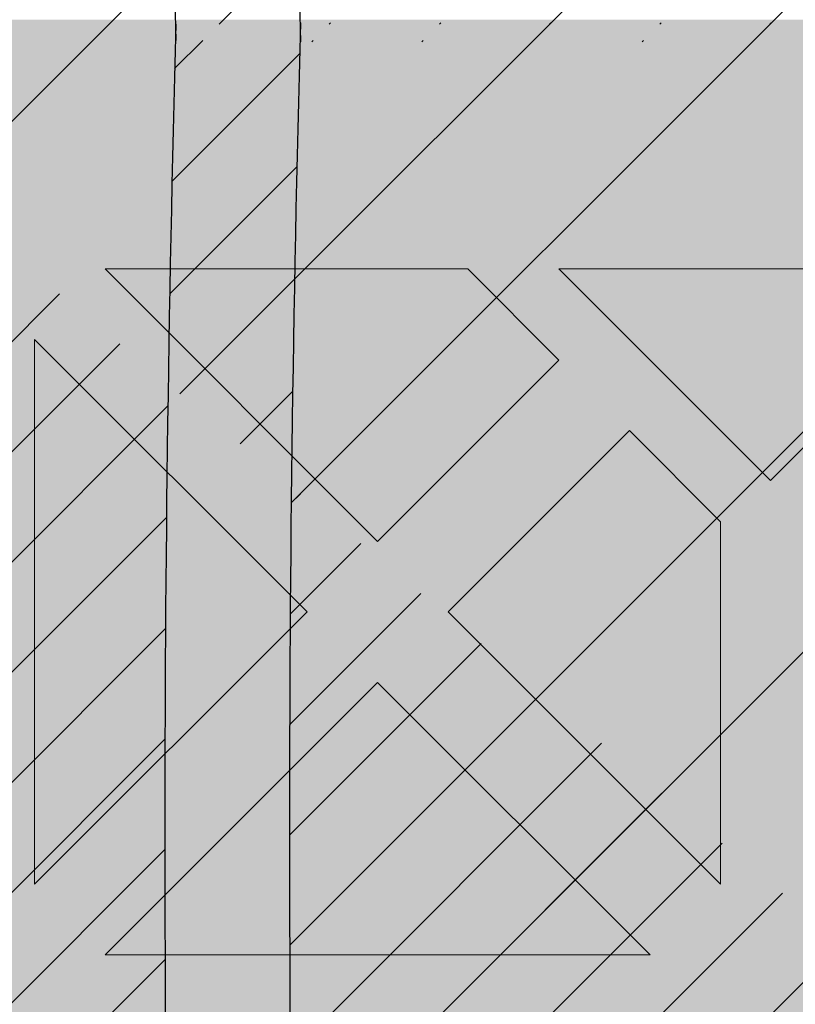
# Model space of a CAD drawing. Units: inches. Extents: x 844 to 2234, y 346 to 1084.
# Tile 11 of 93: x 1120.937 to 1122.921, y 693.702 to 696.22. Entities that reach past the tile are written whole.
import ezdxf

# ---------------------------------------------------------------- set-up
doc = ezdxf.new("R2010")
doc.units = ezdxf.units.IN
doc.header["$MEASUREMENT"] = 0
for name, color, linetype, lineweight in [('A-ANNO-DIMS', 2, 'Continuous', 18), ('furniture', 8, 'Continuous', 18), ('RA-AP-01$0$INT', 35, 'Continuous', 5)]:
    doc.layers.add(name, color=color, linetype=linetype, lineweight=lineweight)
doc.layers.add('RA-AP-01$0$FURN', color=3, linetype='Continuous')
doc.layers.add('RA-AP-01$0$WOOD', color=64, linetype='Continuous')
doc.styles.get("Standard").update_dxf_attribs({"font": 'arial.ttf'})
doc.dimstyles.get("Standard").update_dxf_attribs({"dimtxt": 6, "dimasz": 3, "dimexe": 0.18, "dimexo": 0.0625, "dimgap": 0.09, "dimtad": 0, "dimtih": 1, "dimtoh": 1, "dimdec": 1, "dimzin": 0, "dimdsep": 46, "dimlunit": 3, "dimtxsty": 'Standard', "dimblk": 'ARCHTICK', "dimcen": 0.09, "dimadec": 0, "dimazin": 0, "dimtfac": 1, "dimtdec": 1, "dimtofl": 0, "dimtmove": 0, "dimatfit": 3, "dimfxl": 1, "dimtolj": 1, "dimtzin": 0, "dimarcsym": 0})

# ---------------------------------------------------------------- blocks, each defined once
blk = doc.blocks.new('A$C18D01794')
at = {"layer": 'RA-AP-01$0$INT'}
h = blk.add_hatch(color=256, dxfattribs=at)
h.paths.add_polyline_path([(4.585917135068448, -6.356712009588273), (4.614201406330596, -6.356712009589021), (4.668846067270487, -6.411356670531338), (4.723490728212344, -6.356712009591912), (4.771774999457151, -6.35671200959319), (4.826419660396886, -6.411356670535356), (4.862780050090322, -6.374996280843536), (4.844495778842715, -6.356712009595112), (4.862780050090411, -6.356712009595595), (4.905206456960182, -6.399138416468211), (4.947632863832445, -6.356712009597838), (4.965917135079675, -6.356712009598322), (4.947632863831759, -6.374996280845421), (4.983993253523576, -6.411356670538857), (5.038637914464627, -6.356712009600247), (5.08692218571208, -6.356712009601523), (5.141566846649976, -6.411356670541852), (5.196211507589851, -6.356712009604411), (5.224495778822615, -6.356712009605161), (4.905206456953975, -6.676001331473793)])
h.paths.add_polyline_path([(4.895206456956031, -6.637717060225675), (4.895206456958921, -6.528427738347902), (4.840561796018589, -6.583072399285802)], flags=16)
h.paths.add_polyline_path([(4.915206456955638, -6.637717060226121), (4.969851117895509, -6.583072399288678), (4.915206456957609, -6.528427738348344)], flags=16)
h.paths.add_polyline_path([(4.826419660395175, -6.568930263661755), (4.881064321335613, -6.514285602723745), (4.771774999456703, -6.514285602720857)], flags=16)
h.paths.add_polyline_path([(4.983993253519558, -6.568930263665262), (5.038637914460456, -6.514285602726792), (4.929348592581548, -6.514285602724816)], flags=16)
h.paths.add_polyline_path([(4.881064321336025, -6.494285602723742), (4.826419660397532, -6.439640941782821), (4.771774999457062, -6.494285602720859)], flags=16)
h.paths.add_polyline_path([(4.929348592582019, -6.494285602724817), (5.038637914460982, -6.494285602726792), (4.983993253522945, -6.439640941786327)], flags=16)
h.paths.add_polyline_path([(4.895206456960191, -6.480143467100443), (4.895206456962115, -6.407422687715913), (4.876922185715016, -6.389138416467584), (4.840561796021581, -6.425498806159401)], flags=16)
h.paths.add_polyline_path([(4.915206456958487, -6.480143467100889), (4.969851117899527, -6.425498806162279), (4.933490728206909, -6.389138416468043), (4.9152064569598, -6.40742268771434)], flags=16)
h.paths.add_polyline_path([(4.757632863832376, -6.480143467096812), (4.812277524772842, -6.425498806158772), (4.757632863834348, -6.370854145217844)], flags=16)
h.paths.add_polyline_path([(4.737632863832376, -6.480143467096286), (4.737632863834348, -6.370854145217375), (4.682988202893906, -6.425498806155385)], flags=16)
h.paths.add_polyline_path([(5.05278005008503, -6.480143467103376), (5.052780050087917, -6.370854145224413), (4.998135389146995, -6.425498806162908)], flags=16)
h.paths.add_polyline_path([(5.072780050085024, -6.480143467103744), (5.127424711025931, -6.42549880616527), (5.072780050087916, -6.370854145224832)], flags=16)
h.paths.add_polyline_path([(4.935917135072783, -6.706712009592292), (5.255206456948811, -6.387422687716309), (5.255206456948932, -6.415706958964177), (5.200561796010279, -6.470351619902839), (5.255206456949403, -6.524996280841948), (5.25520645694961, -6.5732805520894), (5.200561796009787, -6.627925213029239), (5.236922185702417, -6.664285602721864), (5.255206456949919, -6.646001331474357), (5.255206456949998, -6.664285602721898), (5.212780050078687, -6.706712009592262), (5.25520645695036, -6.749138416463932), (5.255206456950438, -6.767422687711313), (5.236922185702424, -6.749138416463297), (5.200561796009796, -6.785498806155928), (5.255206456950753, -6.840143467096874), (5.25520645695096, -6.888427738341682), (5.200561796010322, -6.943072399282328), (5.255206456951428, -6.997717060223427), (5.255206456951547, -7.026001331471006)])
h.paths.add_polyline_path([(5.042988202883395, -6.785498806155427), (5.097632863823085, -6.840143467095101), (5.097632863822622, -6.730854145216193)], flags=16)
h.paths.add_polyline_path([(5.028846067259663, -6.771356670531693), (5.083490728198774, -6.716712009592573), (4.974201406321001, -6.716712009593042)], flags=16)
h.paths.add_polyline_path([(5.117632863823087, -6.840143467095186), (5.172277524762331, -6.785498806155926), (5.11763286382262, -6.730854145216225)], flags=16)
h.paths.add_polyline_path([(5.08349072819877, -6.696712009593886), (5.028846067259652, -6.642067348654775), (4.974201406320998, -6.696712009593438)], flags=16)
h.paths.add_polyline_path([(5.131774999446817, -6.854285602718917), (5.186419660386065, -6.799640941779662), (5.241064321325782, -6.854285602719365)], flags=17)
h.paths.add_polyline_path([(5.131774999446228, -6.716712009592374), (5.186419660386065, -6.771356670532194), (5.222780050079488, -6.734996280838764), (5.204495778832781, -6.716712009592063)], flags=16)
h.paths.add_polyline_path([(5.097632863822613, -6.682569873970264), (5.097632863823061, -6.573280552091354), (5.042988202883383, -6.627925213031044)], flags=16)
h.paths.add_polyline_path([(5.131774999446899, -6.874285602718915), (5.241064321325809, -6.874285602719364), (5.186419660386591, -6.928930263658598)], flags=17)
h.paths.add_polyline_path([(5.131774999446226, -6.696712009594078), (5.204495778830767, -6.696712009594374), (5.22278005007868, -6.67842773834687), (5.186419660386049, -6.642067348654249)], flags=16)
h.paths.add_polyline_path([(5.11763286382262, -6.682569873970225), (5.17227752476232, -6.627925213030515), (5.117632863823064, -6.573280552091267)], flags=16)
h.paths.add_polyline_path([(5.186419660386069, -6.613783077405491), (5.241064321325754, -6.559138416465795), (5.131774999446791, -6.559138416466263)], flags=16)
h.paths.add_polyline_path([(5.131774999446872, -6.539138416466263), (5.24106432132578, -6.539138416465794), (5.186419660386554, -6.484493755526573)], flags=16)
h.paths.add_polyline_path([(5.255206456951811, -7.08742268770861), (5.255206456951895, -7.106712009588038), (4.555206456956052, -7.106712009588038), (4.555206456956136, -7.087422687708617), (4.905206456953973, -6.737422687710788)])
h.paths.add_polyline_path([(4.983993253513404, -6.8444937555241), (4.92934859257295, -6.899138416462108), (5.03863791445186, -6.899138416465014)], flags=16)
h.paths.add_polyline_path([(4.969851117889988, -6.83035161990006), (4.915206456952556, -6.775706958960171), (4.915206456949648, -6.884996280837944)], flags=16)
h.paths.add_polyline_path([(4.929348592572535, -6.919138416462105), (4.983993253511019, -6.973783077403037), (5.038637914451496, -6.919138416465012)], flags=16)
h.paths.add_polyline_path([(5.052780050074912, -6.93328055208906), (4.998135389134438, -6.987925213027088), (5.052780050072919, -7.042569873968025)], flags=16)
h.paths.add_polyline_path([(5.07278005007491, -6.933280552089588), (5.072780050072918, -7.042569873968497), (5.127424711013374, -6.987925213030498)], flags=16)
h.paths.add_polyline_path([(4.89520645695295, -6.775706958959721), (4.840561796013067, -6.830351619897157), (4.895206456950961, -6.884996280837494)], flags=16)
h.paths.add_polyline_path([(4.915206456948365, -6.933280552085403), (4.915206456946434, -7.006001331471951), (4.933490728192729, -7.024285602719066), (4.969851117886972, -6.987925213026453)], flags=16)
h.paths.add_polyline_path([(4.881064321327021, -6.899138416461022), (4.82641966038902, -6.84449375552057), (4.771774999448108, -6.899138416459029)], flags=16)
h.paths.add_polyline_path([(4.895206456950073, -6.933280552084951), (4.840561796009022, -6.987925213023558), (4.876922185700835, -7.024285602716997), (4.895206456948749, -7.006001331469487)], flags=16)
h.paths.add_polyline_path([(4.983993253510392, -7.0020673486505), (4.947632863816944, -7.038427738342319), (4.965917135064043, -7.05671200959023), (5.038637914448995, -7.056712009591555)], flags=16)
h.paths.add_polyline_path([(4.881064321326543, -6.91913841646102), (4.771774999447578, -6.919138416459031), (4.826419660385607, -6.973783077399508)], flags=16)
h.paths.add_polyline_path([(4.905206456946447, -7.014285602717636), (4.862780050074785, -7.056712009588352), (4.947632863816685, -7.056712009589775)], flags=16)
h.paths.add_polyline_path([(5.14156684663679, -7.002067348654549), (5.086922185696452, -7.056712009592438), (5.196211507574223, -7.056712009594425)], flags=16)
h.paths.add_polyline_path([(4.8264196603837, -7.002067348646972), (4.771774999442643, -7.056712009585575), (4.8444957788276, -7.056712009587508), (4.862780050075511, -7.038427738340416)], flags=16)
h.paths.add_polyline_path([(4.812277524760289, -6.98792521302292), (4.757632863822258, -6.933280552082447), (4.757632863819352, -7.042569873961408)], flags=16)
h.paths.add_polyline_path([(4.73763286382226, -6.933280552082079), (4.682988202881349, -6.987925213020536), (4.737632863819352, -7.04256987396099)], flags=16)
h.paths.add_polyline_path([(4.723490728195188, -7.056712009584289), (4.668846067257299, -7.002067348643949), (4.614201406317417, -7.056712009581383)], flags=16)
h.paths.add_polyline_path([(4.597632863829262, -6.706712009592262), (4.555206456957951, -6.664285602721896), (4.555206456958029, -6.646001331474357), (4.573490728205535, -6.664285602721864), (4.609851117898167, -6.627925213029238), (4.555206456958338, -6.573280552089402), (4.555206456958546, -6.524996280841952), (4.60985111789767, -6.470351619902839), (4.555206456959015, -6.415706958964177), (4.555206456959138, -6.387422687716309), (4.874495778835167, -6.70671200959229), (4.5552064569564, -7.026001331471015), (4.555206456956523, -6.997717060223433), (4.609851117897629, -6.94307239928233), (4.555206456956988, -6.888427738341681), (4.555206456957198, -6.840143467096881), (4.609851117898153, -6.78549880615593), (4.573490728205528, -6.749138416463297), (4.555206456957507, -6.76742268771132), (4.555206456957585, -6.749138416463933)])
h.paths.add_polyline_path([(4.712780050085332, -6.730854145216195), (4.712780050084863, -6.840143467095105), (4.767424711024555, -6.785498806155427)], flags=16)
h.paths.add_polyline_path([(4.726922185709173, -6.716712009592573), (4.781566846648288, -6.771356670531693), (4.836211507586949, -6.716712009593043)], flags=16)
h.paths.add_polyline_path([(4.692780050085327, -6.730854145216225), (4.638135389145619, -6.785498806155928), (4.692780050084865, -6.840143467095185)], flags=16)
h.paths.add_polyline_path([(4.726922185709182, -6.696712009593886), (4.836211507586949, -6.696712009593436), (4.7815668466483, -6.642067348654773)], flags=16)
h.paths.add_polyline_path([(4.678637914461726, -6.71671200959237), (4.605917135075169, -6.716712009592063), (4.587632863828464, -6.734996280838766), (4.623993253521887, -6.771356670532195)], flags=16)
h.paths.add_polyline_path([(4.712780050085336, -6.68256987397026), (4.767424711024568, -6.627925213031042), (4.71278005008489, -6.573280552091352)], flags=16)
h.paths.add_polyline_path([(4.678637914461726, -6.696712009594076), (4.623993253521899, -6.642067348654247), (4.587632863829271, -6.67842773834687), (4.605917135077185, -6.696712009594376)], flags=16)
h.paths.add_polyline_path([(4.692780050085336, -6.682569873970228), (4.692780050084889, -6.573280552091267), (4.638135389145632, -6.627925213030515)], flags=16)
h.paths.add_polyline_path([(4.623993253521885, -6.799640941779662), (4.678637914461131, -6.854285602718915), (4.56934859258217, -6.854285602719365)], flags=17)
h.paths.add_polyline_path([(4.623993253521901, -6.613783077405509), (4.678637914461158, -6.559138416466263), (4.569348592582195, -6.559138416465795)], flags=16)
h.paths.add_polyline_path([(4.678637914461051, -6.874285602718915), (4.623993253521361, -6.928930263658598), (4.569348592582143, -6.874285602719364)], flags=17)
h.paths.add_polyline_path([(4.678637914461076, -6.539138416466263), (4.623993253521399, -6.484493755526573), (4.569348592582167, -6.539138416465796)], flags=16)
h = blk.add_hatch(color=256, dxfattribs=at)
h.paths.add_polyline_path([(4.895206456952951, -6.77570695895972), (4.840561796013068, -6.830351619897156), (4.895206456950958, -6.884996280837495)])
h.paths.add_polyline_path([(4.915206456949649, -6.884996280837942), (4.969851117889987, -6.830351619900054), (4.915206456952556, -6.775706958960171)])
h.paths.add_polyline_path([(5.038637914451862, -6.899138416465013), (4.983993253513403, -6.8444937555241), (4.929348592572953, -6.899138416462106)])
h.paths.add_polyline_path([(4.929348592572535, -6.919138416462105), (4.983993253511018, -6.973783077403037), (5.038637914451497, -6.919138416465012)])
h.paths.add_polyline_path([(4.915206456948366, -6.933280552085397), (4.915206456946433, -7.006001331471951), (4.93349072819273, -7.024285602719068), (4.969851117886972, -6.987925213026454)])
h.paths.add_polyline_path([(5.038637914448995, -7.056712009591553), (4.983993253510389, -7.002067348650502), (4.947632863816946, -7.038427738342318), (4.965917135064043, -7.05671200959023)])
h.paths.add_polyline_path([(5.05278005007292, -7.042569873968023), (5.05278005007491, -6.933280552089059), (4.998135389134438, -6.987925213027088)])
h.paths.add_polyline_path([(5.07278005007292, -7.042569873968496), (5.127424711013374, -6.987925213030498), (5.072780050074909, -6.933280552089588)])
h.paths.add_polyline_path([(5.141566846636789, -7.002067348654547), (5.086922185696449, -7.056712009592438), (5.196211507574223, -7.056712009594425)])
h.paths.add_polyline_path([(4.947632863816688, -7.056712009589774), (4.905206456946449, -7.014285602717634), (4.862780050074784, -7.056712009588353)])
h.paths.add_polyline_path([(4.840561796009025, -6.987925213023556), (4.876922185700834, -7.024285602716997), (4.895206456948747, -7.006001331469488), (4.895206456950075, -6.933280552084953)])
h.paths.add_polyline_path([(4.88106432132654, -6.919138416461021), (4.771774999447577, -6.919138416459031), (4.826419660385606, -6.973783077399508)])
h.paths.add_polyline_path([(4.881064321327019, -6.899138416461022), (4.826419660389019, -6.844493755520571), (4.771774999448108, -6.89913841645903)])
h.paths.add_polyline_path([(4.757632863819352, -7.042569873961409), (4.812277524760284, -6.987925213022922), (4.757632863822259, -6.933280552082447)])
h.paths.add_polyline_path([(4.8264196603837, -7.002067348646974), (4.771774999442646, -7.056712009585575), (4.844495778827599, -7.05671200958751), (4.862780050075512, -7.038427738340417)])
h.paths.add_polyline_path([(4.737632863819352, -7.042569873960988), (4.737632863822258, -6.933280552082078), (4.682988202881349, -6.987925213020538)])
h.paths.add_polyline_path([(4.668846067257299, -7.002067348643952), (4.61420140631742, -7.056712009581384), (4.723490728195189, -7.056712009584292)])
for p, q in [((4.771774999447578, -6.919138416459031), (4.881064321326541, -6.919138416461022)), ((4.771774999447578, -6.919138416459031), (4.826419660385606, -6.973783077399508)), ((4.881064321326541, -6.919138416461022), (4.826419660385606, -6.973783077399508)), ((4.757632863822258, -6.933280552082445), (4.812277524760285, -6.987925213022922)), ((4.757632863822258, -6.933280552082445), (4.757632863819352, -7.042569873961408)), ((4.895206456950073, -6.933280552084951), (4.840561796009024, -6.987925213023556)), ((4.895206456948748, -7.006001331469903), (4.895206456950073, -6.933280552084951)), ((4.757632863819352, -7.042569873961408), (4.812277524760285, -6.987925213022922)), ((4.840561796009024, -6.987925213023554), (4.876922185700835, -7.024285602716997)), ((4.771774999442645, -7.056712009585574), (4.8264196603837, -7.002067348646972)), ((4.826419660383698, -7.002067348646972), (4.862780050075511, -7.038427738340416)), ((4.895206456946431, -7.006001331471805), (4.876922185700835, -7.024285602716997)), ((4.905206456946449, -7.014285602717635), (4.862780050074783, -7.056712009588354)), ((4.905206456946449, -7.014285602717635), (4.94763286381669, -7.056712009589775)), ((4.844495778827597, -7.056712009587512), (4.862780050075513, -7.038427738340416)), ((4.844495778827597, -7.05671200958751), (4.771774999442645, -7.056712009585574)), ((4.94763286381669, -7.056712009589775), (4.862780050074783, -7.056712009588354))]:
    blk.add_line(p, q, dxfattribs=at)
blk = doc.blocks.new('A$C32926AE1')
at = {"layer": 'RA-AP-01$0$FURN'}
h = blk.add_hatch(dxfattribs=at)
h.set_pattern_fill('ANSI31', color=256, scale=0.1, style=0)
h.set_pattern_definition([(45, (0, 0), (-0.0088388347648318, 0.0088388347648318), [])])
edge = h.paths.add_edge_path(flags=16)
edge.add_arc((4.904771284329206, 4.246793130718756), 0.2603971832811541, 75.22398030683196, 104.7760196931204)
edge.add_arc((4.904771284329206, 4.246793130718756), 0.2603971832811541, 75.223980306832, 104.77601969312039, ccw=False)
edge = h.paths.add_edge_path(flags=16)
edge.add_arc((4.904771284329206, 4.067062675376612), 0.2603971832811541, 255.2239803068796, 284.776019693168)
edge.add_arc((4.904771284329206, 4.067062675376612), 0.2603971832811541, 255.22398030687958, 284.77601969316805, ccw=False)
edge = h.paths.add_edge_path(flags=0)
edge.add_arc((4.904771284329206, 4.067062675376612), 0.2603971832811541, 255.2239803068796, 284.776019693168)
edge.add_arc((4.904771284329206, 4.067062675376612), 0.2603971832811541, 255.22398030687958, 284.77601969316805, ccw=False)
edge = h.paths.add_edge_path(flags=0)
edge.add_arc((4.904771284329206, 4.067062675376612), 0.2603971832811541, 255.2239803068796, 284.776019693168)
edge.add_arc((4.904771284329206, 4.067062675376612), 0.2603971832811541, 255.22398030687958, 284.77601969316805, ccw=False)
edge = h.paths.add_edge_path()
edge.add_arc((4.604388392048174, 4.588829985554312), 0.1599999999999918, 342.3781640246255, 354.4317409793762)
edge.add_arc((5.090145208887507, 4.43216705527679), 0.3503971832811637, 162.0091218307731, 180.3186872093483)
edge.add_arc((5.205154176610243, 4.588829985554953), 0.1599999999999917, 185.5682590208461, 197.6218359767349)
edge.add_arc((4.904771284329229, 4.246793130718735), 0.3503971832811761, 72.00912183053516, 107.9908781690354)
edge.add_arc((9.535952835716557, 4.28682295566602), 4.798342501046485, 178.2875002453811, 181.5576802719453)
edge.add_arc((4.719397359771122, 4.43216705527679), 0.3503971832811637, 359.6813127906516, 377.9908781692269)
edge.add_arc((9.535967292294904, 4.286822350292874), 4.778371420254705, 178.2965938931842, 181.5667745797229)
edge.add_arc((4.719397359771122, 4.43216705527679), 0.3303971832811637, 359.6813127906516, 377.9908781692269)
edge.add_arc((0.2735752763637294, 4.286822350292874), 4.7783714202547, 358.4332254202771, 361.7034061068158)
edge.add_arc((5.061434214606998, 4.732549947558029), 0.1600000000000254, 252.3781640250584, 264.4317409792362)
edge.add_arc((4.748108354051257, 4.732549947558012), 0.1600000000000541, 275.5682590208426, 287.6218359759532)
edge.add_arc((4.604388392048115, 4.588829985554317), 0.1800000000000505, 342.3567572500182, 349.3735009646207)
edge.add_arc((5.205154176610254, 4.588829985554976), 0.1800000000000069, 190.6264990356027, 197.6432427513933)
edge.add_arc((5.061434214607106, 4.732549947558013), 0.1800000000000424, 252.3567572496606, 259.3735009644582)
edge.add_arc((4.904771284329208, 4.246793130718737), 0.3303971832811676, 71.99844483668534, 108.0015551637021)
edge.add_arc((4.748108354051414, 4.732549947558045), 0.1800000000000547, 280.6264990355479, 287.6432427495938)
edge.add_arc((5.090145208887514, 4.432167055276789), 0.2803971832811691, 162.8706300666893, 180.816523289902)
edge.add_arc((4.719397359771136, 4.432167055276689), 0.2803971832811534, 359.183476710103, 377.1293699333214)
edge.add_arc((4.904771284329222, 4.246793130718737), 0.2803971832811769, 72.87063006672916, 107.1293699332334)
edge.add_arc((5.090145208887522, 4.432167055276788), 0.2603971832811776, 165.2239803068007, 180.9953123810312)
edge.add_arc((4.719397359771141, 4.432167055276699), 0.2603971832811458, 359.0046876189768, 374.7760196932087)
edge.add_arc((5.090145208887507, 4.43216705527679), 0.3303971832811637, 162.0091218307731, 180.3186872093483)
edge.add_arc((9.53595427642584, 4.285015535491528), 4.728345371032053, 178.265043920078, 181.5679956281801)
edge.add_arc((0.2735882922327999, 4.285015535491582), 4.728345371032045, 358.4320043718193, 361.7349560799204)
edge.add_arc((9.535953591267507, 4.284458026472751), 4.708343996644348, 178.2573054306777, 181.5704995759608)
edge.add_arc((0.273588977391114, 4.284458026472785), 4.708343996644358, 358.4295004240388, 361.7426945693213)
edge.add_arc((0.2735889773911131, 4.029397779622582), 4.708343996644359, 358.2573054306787, 361.5704995759613)
edge.add_arc((9.535953591267518, 4.029397779622618), 4.708343996644359, 178.4295004240391, 181.7426945693223)
edge.add_arc((0.2735882922327901, 4.028840270603786), 4.728345371032054, 358.2650439200796, 361.5679956281808)
edge.add_arc((9.53595427642584, 4.028840270603841), 4.728345371032054, 178.4320043718199, 181.7349560799219)
edge.add_arc((0.2735752763637302, 4.027033455802493), 4.778371420254699, 358.2965938931842, 361.5667745797229)
edge.add_arc((4.719397359771122, 3.881688750818578), 0.3303971832811637, 342.0091218307731, 360.3186872093484)
edge.add_arc((5.090145208887507, 3.881688750818578), 0.3303971832811637, 179.6813127906516, 197.9908781692269)
edge.add_arc((9.535967292294904, 4.027033455802493), 4.778371420254705, 178.433225420277, 181.7034061068158)
edge.add_arc((4.719397359771122, 3.881688750818578), 0.3503971832811637, 342.0091218307731, 360.3186872093484)
edge.add_arc((9.53595283571655, 4.027032850429349), 4.79834250104648, 178.4423197280546, 181.7124997546188)
edge.add_arc((4.719397359771141, 3.881688750818669), 0.2603971832811458, 345.2239803067913, 360.9953123810232)
edge.add_arc((5.090145208887522, 3.88168875081858), 0.2603971832811776, 179.0046876189687, 194.7760196931993)
edge.add_arc((4.904771284329222, 4.067062675376631), 0.2803971832811769, 252.8706300667665, 287.1293699332708)
edge.add_arc((4.719397359771136, 3.881688750818678), 0.2803971832811534, 342.8706300666787, 360.8165232898969)
edge.add_arc((5.090145208887514, 3.881688750818579), 0.2803971832811691, 179.183476710098, 197.1293699333106)
edge.add_arc((4.748108354051414, 3.581305858537323), 0.1800000000000547, 72.3567572504062, 79.37350096445199)
edge.add_arc((4.904771284329208, 4.067062675376631), 0.3303971832811676, 251.9984448362979, 288.0015551633146)
edge.add_arc((5.061434214607106, 3.581305858537355), 0.1800000000000424, 100.6264990355418, 107.6432427503394)
edge.add_arc((5.205154176610254, 3.725025820540392), 0.1800000000000069, 162.3567572486066, 169.3735009643972)
edge.add_arc((4.604388392048115, 3.725025820541051), 0.1800000000000505, 10.62649903537925, 17.64324274998182)
edge.add_arc((4.748108354051257, 3.581305858537356), 0.1600000000000541, 72.37816402404681, 84.43174097915735)
edge.add_arc((4.904771284329229, 4.067062675376632), 0.3503971832811761, 252.0091218309645, 287.9908781694648)
edge.add_arc((5.061434214606998, 3.581305858537339), 0.1600000000000254, 95.56825902076373, 107.6218359749416)
edge.add_arc((5.205154176610243, 3.725025820540414), 0.1599999999999917, 162.3781640232651, 174.4317409791539)
edge.add_arc((5.090145208887507, 3.881688750818578), 0.3503971832811637, 179.6813127906516, 197.9908781692269)
edge.add_arc((4.604388392048174, 3.725025820541056), 0.1599999999999918, 5.568259020623824, 17.62183597537444)
edge.add_arc((0.2735897329420762, 4.28682295566602), 4.798342501046482, 358.4423197280547, 361.7124997546188)
edge.add_arc((0.2735897329420691, 4.027032850429348), 4.798342501046489, 358.2875002453812, 361.5576802719453)
at = {"layer": 'RA-AP-01$0$WOOD'}
h = blk.add_hatch(color=256, dxfattribs=at)
h.dxf.hatch_style = 1
h.paths.add_polyline_path([(5.157430609644524, 4.573483066760929, -0.1009492694046607), (5.155401577623758, 4.593365984175333, -0.1842662638101597), (5.172249623284174, 4.638795604568598, 0.2056608120311276), (5.179560981299304, 4.661316324430096, 0.3614336704623542), (5.134352340494423, 4.706524965234944, 0.2056608120311297), (5.111831620632933, 4.699213607219793, -0.1842662638101113), (5.066402000239693, 4.682365561559342, -0.1055311479399994), (5.045656153913092, 4.68467289944697, 0.1567636581983829), (4.763886414745334, 4.684672899446966, -0.1055311479399895), (4.743140568418733, 4.68236556155934, -0.1842662638100833), (4.6977109480255, 4.69921360721979, 0.2056608120302612), (4.675190228164109, 4.706524965234949, 0.3614336704708441), (4.629981587358889, 4.66131632442871, 0.2056608120245944), (4.637292945374126, 4.638795604567974, -0.1842662638101024), (4.654140991034615, 4.59336598417475, -0.1009492694055169), (4.652111959013835, 4.573483066760181, 0.021410119221476), (4.629748025606143, 4.156712009541676, 0.0214101192214795), (4.652111959013809, 3.739940952323101, -0.1009492694059586), (4.654140991034615, 3.720058034908448, -0.1842662638100975), (4.637292945374126, 3.674628414515226, 0.2056608120245705), (4.629981587358889, 3.652107694654492, 0.3614336704708879), (4.675190228164113, 3.606899053848249, 0.2056608120302384), (4.697710948025501, 3.614210411863408, -0.1842662638100995), (4.743140568418738, 3.63105845752386, -0.1055311479402541), (4.763886414745388, 3.628751119636215, 0.1567636581983776), (5.045656153913137, 3.628751119636244, -0.1055311479397538), (5.066402000239692, 3.631058457523857, -0.1842662638101067), (5.111831620632931, 3.614210411863407, 0.2056608120310924), (5.134352340494417, 3.606899053848256, 0.3614336704624001), (5.179560981299307, 3.652107694653103, 0.2056608120311314), (5.172249623284175, 3.6746284145146, -0.1842662638101402), (5.155401577623758, 3.72005803490786, -0.1009492694051366), (5.15743060964455, 3.739940952322354, 0.0214101192215073), (5.179794543052287, 4.156712009541468, 0.0214101192215252)])
h.paths.add_polyline_path([(4.639748609479751, 4.156712009541513, 0.0213537860821624), (4.661970494867118, 3.741887061152232, -0.094075836301374), (4.664143710413708, 3.7196126951003, -0.1824818158568985), (4.644813765429836, 3.668037719127816, 0.2056608120245319), (4.639939526753007, 3.653023905887301, 0.3614336704710246), (4.676106439397173, 3.616856993242342, 0.2056608120302234), (4.691120252638095, 3.621731231919122, -0.1824818158602558), (4.742695228611606, 3.641061176902986, -0.1029891339458722), (4.766991894714349, 3.638256818950944, 0.156709409989566), (5.042550673941472, 3.638256818950105, -0.102989133958497), (5.066847340047078, 3.641061176902949, -0.1824818158594995), (5.118422316020358, 3.621731231919103, 0.2056608120311416), (5.133436129261316, 3.616856993242346, 0.3614336704621468), (5.169603041905217, 3.653023905886178, 0.2056608120310986), (5.164728803228477, 3.668037719127177, -0.1824818158565612), (5.145398858244737, 3.719612695099578, -0.0940758363009313), (5.147572073791232, 3.741887061151398, 0.0213537860822023), (5.169793959178681, 4.156712009541451, 0.0213537860822226), (5.147572073791203, 4.571536957931898, -0.0940758363005034), (5.145398858244737, 4.59381132398362, -0.1824818158565587), (5.164728803228476, 4.645386299956021, 0.2056608120311045), (5.169603041905216, 4.66040011319702, 0.3614336704621845), (5.133436129261313, 4.696567025840856, 0.2056608120310773), (5.118422316020359, 4.691692787164098, -0.182481815859508), (5.066847340047078, 4.67236284218025, -0.1029891339584606), (5.04255067394148, 4.675167200133092, 0.156709409989566), (4.766991894714357, 4.675167200132257, -0.1029891339458842), (4.742695228611611, 4.672362842180213, -0.1824818158602725), (4.691120252638095, 4.691692787164077, 0.2056608120302152), (4.676106439397174, 4.696567025840858, 0.3614336704710363), (4.639939526753005, 4.660400113195899, 0.2056608120245495), (4.644813765429837, 4.645386299955384, -0.1824818158568934), (4.664143710413708, 4.593811323982902, -0.0940758363009187), (4.661970494867149, 4.571536957931074, 0.021353786082177)], flags=16)
h.paths.add_polyline_path([(5.129794543052235, 4.432167055276933, -0.0141661062790638), (5.130152669293814, 4.156927903047693, -0.0141661062790647), (5.129794543052234, 3.881688750818433, -0.0785247771143638), (5.10979738006795, 3.755143611847103, 0.0945969212073497), (5.105408519571111, 3.717898134952927, 0.1043170707844957), (5.116074640131521, 3.670385395016088, 0.1043170707864965), (5.068561900193738, 3.681051515576561, 0.09459692119553), (5.031316423304057, 3.676662655080835, -0.1580239521427272), (4.778226145355827, 3.676662655080367, 0.0945969211986668), (4.740980668464973, 3.681051515576592, 0.1043170707882822), (4.693467928526415, 3.670385395015844, 0.1043170707867916), (4.704134049087309, 3.717898134953662, 0.0945969211972894), (4.69974518859162, 3.755143611844042, -0.0785247771163196), (4.679748025606343, 3.881688750818406, -0.0141661062790663), (4.679389899364763, 4.156927903047693, -0.0141661062790672), (4.679748025606343, 4.432167055276998, -0.0785247771163064), (4.699745188591625, 4.55871219425134, 0.094596921197333), (4.704134049087308, 4.595957671141738, 0.1043170707867205), (4.693467928526416, 4.643470411079523, 0.1043170707882628), (4.740980668464965, 4.632804290518776, 0.0945969211988114), (4.778226145355874, 4.637193151015016, -0.158023952142669), (5.031316423304015, 4.637193151014546, 0.0945969211956361), (5.068561900193736, 4.632804290518806, 0.1043170707864979), (5.11607464013152, 4.643470411079278, 0.1043170707844617), (5.105408519571112, 4.595957671142455, 0.0945969212074597), (5.109797380067959, 4.558712194248236, -0.0785247771143467)], flags=0)
h.paths.add_polyline_path([(5.119794532311105, 4.432259799204851, -0.0142000800617244), (5.120156169157484, 4.156927903047701, -0.0142000800617277), (5.119794532311105, 3.881596006890482, -0.0784894509520253), (5.100273383573699, 3.758192358677797, 0.0940138827242913), (5.095413455884425, 3.717477693979438, 0.0606271852308753), (5.099615656341024, 3.686844378806616, 0.0606271852322524), (5.068982341167493, 3.691046579263239, 0.0940138827010453), (5.028267676478798, 3.686186651576848, -0.1580706864508061), (4.781274892180912, 3.686186651576435, 0.0940138827026903), (4.740560227491556, 3.691046579263279, 0.0606271852339895), (4.709926912317155, 3.686844378806508, 0.0606271852329405), (4.714129112773991, 3.717477693980356, 0.094013882701304), (4.709269185087677, 3.758192358669163, -0.0784894509577193), (4.689748036347473, 3.881596006890469, -0.014200080061729), (4.689386399501094, 4.156927903047709, -0.0142000800617217), (4.689748036347473, 4.432259799204808, -0.078489450957724), (4.709269185087651, 4.555663447426125, 0.0940138827014585), (4.714129112773992, 4.596378112114996, 0.0606271852329731), (4.709926912317154, 4.62701142728886, 0.0606271852340196), (4.74056022749157, 4.622809226832087, 0.0940138827024997), (4.781274892180847, 4.627669154518912, -0.1580706864508359), (5.028267676478777, 4.627669154518526, 0.0940138827010946), (5.068982341167492, 4.622809226832129, 0.060627185232254), (5.099615656341024, 4.627011427288751, 0.0606271852308727), (5.095413455884425, 4.59637811211593, 0.0940138827241088), (5.100273383573675, 4.555663447417647, -0.0784894509520978)], flags=0)
h.paths.add_polyline_path([(5.06978912287499, 4.430218106756144, -0.014241683694547), (5.070173729147532, 4.156927903047672, -0.0142416836945458), (5.06978912287499, 3.883637699339223, -0.0800609523125196), (5.052662118612511, 3.773463122773442, 0.0526421978001116), (5.04590916754064, 3.740550867606997, 0.0526421977992423), (5.012996912374707, 3.73379791653534, -0.1583028414718258), (4.796545656286308, 3.73379791653451, 0.0526421978034211), (4.763633401117837, 3.740550867607021, 0.0526421978018622), (4.756880450045755, 3.773463122774558, -0.0800609523117106), (4.739753445783639, 3.883637699339268, -0.0142416836945435), (4.739368839511098, 4.156927903047671, -0.0142416836945477), (4.739753445783639, 4.430218106756155, -0.0800609523116345), (4.75688045004574, 4.540392683320762, 0.052642197801941), (4.763633401117837, 4.573304938488346, 0.0526421978035071), (4.796545656286361, 4.580057889560873, -0.1583028414717561), (5.012996912374669, 4.580057889560039, 0.0526421977993048), (5.04590916754064, 4.57330493848837, 0.0526421978002057), (5.052662118612529, 4.540392683321868, -0.080060952312477)], flags=0)
h.paths.add_polyline_path([(5.049789715110557, 4.43038092723357, -0.0143097550741839), (5.05018085590259, 4.156927903047715, -0.0143097550741854), (5.049789715110558, 3.883474878861827, -0.0800685599149176), (5.03362098255317, 3.779581877367999, 0.0306258898956367), (5.028241146483733, 3.758218888663947, 0.0306258898977031), (5.006878157778253, 3.75283905259408, -0.1583983521624096), (4.802664410878162, 3.752839052594731, 0.0306258898946014), (4.781301422174808, 3.758218888663924, 0.0306258898967912), (4.775921586105202, 3.779581877368794, -0.080068559914251), (4.759752853548071, 3.883474878861786, -0.0143097550741854), (4.759361712756037, 4.156927903047671, -0.0143097550741854), (4.759752853548071, 4.430380927233557, -0.0800685599142479), (4.775921586105193, 4.534273928726546, 0.0306258898968306), (4.781301422174808, 4.555636917431444, 0.0306258898945754), (4.802664410878143, 4.561016753500631, -0.1583983521624168), (5.006878157778244, 4.561016753501291, 0.0306258898977177), (5.028241146483733, 4.555636917431421, 0.0306258898958182), (5.03362098255321, 4.534273928727244, -0.080068559914796)], flags=0)
h.paths.add_polyline_path([(4.999766070382627, 4.428171244713864, -0.0143443147609634), (5.000198441819402, 4.156927903047689, -0.0143443147609612), (4.999766070382627, 3.885684561381556, -0.0784641635803329), (4.987356730658798, 3.799103304488872, -0.1506053783831347), (4.822185837999821, 3.79910330448882, -0.0784641635803318), (4.809776498276007, 3.885684561381509, -0.014344314760963), (4.809344126839227, 4.156927903047677, -0.0143443147609645), (4.809776498276007, 4.428171244713873, -0.0784641635803192), (4.822185837999822, 4.514752501606549, -0.1506053783831338), (4.987356730658798, 4.514752501606494, -0.078464163580285)], flags=0)
h.paths.add_polyline_path([(4.979755254238824, 4.42764379880488, -0.0143772539198268), (4.980205517789977, 4.156927903047693, -0.0143772539198275), (4.979755254238824, 3.886212007290489, -0.0689242507424422), (4.971183264704897, 3.815276770442801, -0.1296645318904179), (4.838359303953726, 3.815276770442746, -0.0689242507424186), (4.829787314419809, 3.886212007290419, -0.0143772539198292), (4.829337050868653, 4.156927903047653, -0.0143772539198325), (4.829787314419809, 4.427643798804946, -0.0689242507424211), (4.838359303953725, 4.498579035652621, -0.1296645318904187), (4.971183264704897, 4.498579035652565, -0.0689242507424401)], flags=0)
h = blk.add_hatch(color=256, dxfattribs=at)
h.dxf.hatch_style = 1
h.paths.add_polyline_path([(5.145398858244737, 4.59381132398362, -0.1824818158565616), (5.164728803228476, 4.645386299956021, 0.2056608120311045), (5.169603041905216, 4.66040011319702, 0.3614336704621845), (5.133436129261313, 4.696567025840856, 0.2056608120310773), (5.118422316020359, 4.691692787164098, -0.182481815859508), (5.066847340047078, 4.67236284218025, -0.1029891339584606), (5.04255067394148, 4.675167200133092, 0.156709409989566), (4.766991894714357, 4.675167200132257, -0.1029891339458842), (4.742695228611611, 4.672362842180213, -0.1824818158602725), (4.691120252638095, 4.691692787164077, 0.2056608120302152), (4.676106439397174, 4.696567025840858, 0.3614336704710363), (4.639939526753005, 4.660400113195899, 0.2056608120245495), (4.644813765429837, 4.645386299955384, -0.1824818158568934), (4.664143710413708, 4.593811323982902, -0.0940758363009187), (4.661970494867149, 4.571536957931074, 0.0213537860821772), (4.639748609479751, 4.156712009541507, 0.0213537860821625), (4.661970494867119, 3.741887061152226, -0.0940758363013071), (4.664143710413708, 3.719612695100309, -0.1824818158569294), (4.644813765429836, 3.668037719127816, 0.2056608120245319), (4.639939526753007, 3.653023905887301, 0.3614336704710246), (4.676106439397173, 3.616856993242342, 0.2056608120302234), (4.691120252638095, 3.621731231919122, -0.1824818158602558), (4.742695228611606, 3.641061176902986, -0.1029891339458722), (4.766991894714349, 3.638256818950944, 0.156709409989566), (5.042550673941472, 3.638256818950105, -0.102989133958497), (5.066847340047078, 3.641061176902949, -0.1824818158594995), (5.118422316020358, 3.621731231919103, 0.2056608120311416), (5.133436129261316, 3.616856993242346, 0.3614336704621468), (5.169603041905217, 3.653023905886178, 0.2056608120310986), (5.164728803228477, 3.668037719127177, -0.1824818158565612), (5.145398858244737, 3.719612695099578, -0.0940758363009313), (5.147572073791232, 3.741887061151398, 0.0213537860822023), (5.169793959178681, 4.156712009541451, 0.0213537860822226), (5.147572073791203, 4.571536957931898, -0.0940758363004996)])
h.paths.add_polyline_path([(5.109797380067958, 4.55871219424824, -0.0785247771143472), (5.129794543052234, 4.432167055276936, -0.0141661062790644), (5.130152669293814, 4.156927903047685, -0.014166106279066), (5.129794543052234, 3.881688750818401, -0.0785247771143517), (5.109797380067946, 3.755143611847092, 0.0945969212073132), (5.105408519571111, 3.717898134952929, 0.1043170707844995), (5.116074640131521, 3.670385395016088, 0.1043170707864965), (5.068561900193738, 3.681051515576561, 0.09459692119553), (5.031316423304057, 3.676662655080835, -0.1580239521427272), (4.778226145355827, 3.676662655080367, 0.0945969211986668), (4.740980668464973, 3.681051515576592, 0.1043170707882822), (4.693467928526415, 3.670385395015844, 0.1043170707867916), (4.704134049087309, 3.717898134953662, 0.0945969211972894), (4.69974518859162, 3.755143611844042, -0.0785247771163196), (4.679748025606343, 3.881688750818406, -0.0141661062790663), (4.679389899364763, 4.156927903047693, -0.0141661062790672), (4.679748025606343, 4.432167055276998, -0.0785247771163064), (4.699745188591625, 4.55871219425134, 0.094596921197333), (4.704134049087308, 4.595957671141738, 0.1043170707867205), (4.693467928526416, 4.643470411079523, 0.1043170707882628), (4.740980668464965, 4.632804290518776, 0.0945969211988114), (4.778226145355874, 4.637193151015016, -0.158023952142669), (5.031316423304015, 4.637193151014546, 0.0945969211956361), (5.068561900193736, 4.632804290518806, 0.1043170707864979), (5.11607464013152, 4.643470411079278, 0.1043170707844617), (5.105408519571112, 4.595957671142455, 0.0945969212074504)], flags=16)
h.paths.add_polyline_path([(5.100273383573655, 4.55566344741771, -0.0784894509521388), (5.119794532311105, 4.432259799204852, -0.0142000800617252), (5.120156169157484, 4.156927903047686, -0.014200080061726), (5.119794532311105, 3.881596006890502, -0.0784894509520446), (5.100273383573696, 3.758192358677786, 0.0940138827242721), (5.095413455884425, 3.717477693979436, 0.0606271852308692), (5.099615656341024, 3.686844378806616, 0.0606271852322522), (5.068982341167493, 3.691046579263239, 0.0940138827010453), (5.028267676478798, 3.686186651576848, -0.1580706864508061), (4.781274892180912, 3.686186651576435, 0.0940138827026903), (4.740560227491556, 3.691046579263279, 0.0606271852339895), (4.709926912317155, 3.686844378806508, 0.0606271852329405), (4.714129112773991, 3.717477693980356, 0.094013882701304), (4.709269185087677, 3.758192358669163, -0.0784894509577193), (4.689748036347473, 3.881596006890469, -0.014200080061729), (4.689386399501094, 4.156927903047709, -0.0142000800617217), (4.689748036347473, 4.432259799204808, -0.078489450957724), (4.709269185087651, 4.555663447426125, 0.0940138827014585), (4.714129112773992, 4.596378112114996, 0.0606271852329731), (4.709926912317154, 4.62701142728886, 0.0606271852340196), (4.74056022749157, 4.622809226832087, 0.0940138827024997), (4.781274892180847, 4.627669154518912, -0.1580706864508359), (5.028267676478777, 4.627669154518526, 0.0940138827010946), (5.068982341167492, 4.622809226832129, 0.060627185232254), (5.099615656341024, 4.627011427288751, 0.0606271852308727), (5.095413455884425, 4.59637811211593, 0.094013882723957)], flags=0)
h.paths.add_polyline_path([(5.04590916754064, 4.57330493848837, 0.0526421978002057), (5.052662118612529, 4.540392683321868, -0.0800609523124783), (5.06978912287499, 4.430218106756142, -0.0142416836945469), (5.070173729147532, 4.156927903047672, -0.0142416836945458), (5.06978912287499, 3.883637699339223, -0.0800609523125196), (5.052662118612511, 3.773463122773442, 0.0526421978001116), (5.04590916754064, 3.740550867606997, 0.0526421977992423), (5.012996912374707, 3.73379791653534, -0.1583028414718258), (4.796545656286308, 3.73379791653451, 0.0526421978034211), (4.763633401117837, 3.740550867607021, 0.0526421978018622), (4.756880450045755, 3.773463122774558, -0.0800609523117106), (4.739753445783639, 3.883637699339268, -0.0142416836945435), (4.739368839511098, 4.156927903047671, -0.0142416836945477), (4.739753445783639, 4.430218106756155, -0.0800609523116345), (4.75688045004574, 4.540392683320762, 0.052642197801941), (4.763633401117837, 4.573304938488346, 0.0526421978035071), (4.796545656286361, 4.580057889560873, -0.1583028414717561), (5.012996912374669, 4.580057889560039, 0.0526421977993048)], flags=0)
h.paths.add_polyline_path([(5.028241146483733, 4.555636917431422, 0.0306258898956949), (5.033620982553182, 4.534273928727329, -0.0800685599148649), (5.049789715110557, 4.430380927233569, -0.0143097550741839), (5.05018085590259, 4.156927903047715, -0.0143097550741854), (5.049789715110558, 3.883474878861827, -0.0800685599149176), (5.03362098255317, 3.779581877367999, 0.0306258898956367), (5.028241146483733, 3.758218888663947, 0.0306258898977031), (5.006878157778253, 3.75283905259408, -0.1583983521624096), (4.802664410878162, 3.752839052594731, 0.0306258898946014), (4.781301422174808, 3.758218888663924, 0.0306258898967912), (4.775921586105202, 3.779581877368794, -0.080068559914251), (4.759752853548071, 3.883474878861786, -0.0143097550741854), (4.759361712756037, 4.156927903047671, -0.0143097550741854), (4.759752853548071, 4.430380927233557, -0.0800685599142479), (4.775921586105193, 4.534273928726546, 0.0306258898968306), (4.781301422174808, 4.555636917431444, 0.0306258898945754), (4.802664410878143, 4.561016753500631, -0.1583983521624168), (5.006878157778244, 4.561016753501291, 0.0306258898977174)], flags=0)
h.paths.add_polyline_path([(4.987356730658798, 4.514752501606494, -0.0784641635803018), (4.999766070382627, 4.428171244713845, -0.0143443147609637), (5.000198441819402, 4.156927903047665, -0.0143443147609622), (4.999766070382628, 3.885684561381514, -0.0784641635802952), (4.987356730658797, 3.799103304488872, -0.1506053783831338), (4.822185837999821, 3.799103304488819, -0.0784641635803342), (4.809776498276007, 3.885684561381512, -0.0143443147609628), (4.809344126839227, 4.156927903047676, -0.0143443147609646), (4.809776498276007, 4.428171244713873, -0.0784641635803192), (4.822185837999822, 4.514752501606549, -0.1506053783831338)], flags=0)
h.paths.add_polyline_path([(4.971183264704897, 4.498579035652566, -0.0689242507424384), (4.979755254238824, 4.427643798804883, -0.0143772539198276), (4.980205517789977, 4.15692790304768, -0.0143772539198258), (4.979755254238823, 3.88621200729051, -0.0689242507424628), (4.971183264704897, 3.815276770442801, -0.129664531890417), (4.838359303953726, 3.815276770442746, -0.0689242507424186), (4.829787314419809, 3.886212007290419, -0.0143772539198292), (4.829337050868653, 4.156927903047653, -0.0143772539198325), (4.829787314419809, 4.427643798804946, -0.0689242507424211), (4.838359303953725, 4.498579035652621, -0.1296645318904187)], flags=0)
h = blk.add_hatch(dxfattribs=at)
h.set_pattern_fill('ANSI31', color=256, scale=0.05, style=0)
h.set_pattern_definition([(45, (0, 0), (-0.0044194173824159, 0.0044194173824159), [])])
h.paths.add_polyline_path([(5.130152669293814, 4.156927903047704, 0.0141661062790657), (5.129794543052234, 4.432167055276982, 0.0777827904001433), (5.110168979996553, 4.557559993161921, -0.0976515123401879), (5.105408519571111, 4.595957671142454, -0.1043170707844687), (5.116074640131522, 4.64347041107928), (5.099615656341024, 4.627011427288751, 0.0606271852308727), (5.095413455884425, 4.59637811211593, 0.0940138827241088), (5.100273383573675, 4.555663447417647, -0.0784894509520972), (5.119794532311105, 4.432259799204852, -0.0142000800617252), (5.120156169157484, 4.156927903047686, -0.014200080061726), (5.119794532311105, 3.881596006890502, -0.0784894509520446), (5.100273383573696, 3.758192358677786, 0.0940138827242721), (5.095413455884425, 3.717477693979436, 0.0606271852308692), (5.099615656341024, 3.686844378806616), (5.116074640131519, 3.67038539501609, -0.1043170707844594), (5.105408519571112, 3.717898134952912, -0.0976515123401594), (5.11016897999655, 3.756295812933435, 0.0777827904001654), (5.129794543052234, 3.881688750818409, 0.0141661062790665)])
h.paths.add_polyline_path([(5.030164222210597, 3.676291055149937, -0.0976515123472002), (5.068561900193739, 3.681051515576561, -0.1043170707864927), (5.116074640131521, 3.670385395016088), (5.099615656341024, 3.686844378806616, 0.0606271852322522), (5.068982341167493, 3.691046579263239, 0.0940138827010453), (5.028267676478798, 3.686186651576848, -0.1580706864508061), (4.781274892180912, 3.686186651576435, 0.0940138827026903), (4.740560227491556, 3.691046579263279, 0.0606271852339913), (4.709926912317154, 3.686844378806508), (4.693467928526416, 3.670385395015845, -0.1043170707882796), (4.740980668464973, 3.681051515576592, -0.0976515123427246), (4.779378346446416, 3.676291055150394, 0.156512506893803)])
h.paths.add_polyline_path([(4.689748036347473, 3.881596006890472, -0.014200080061729), (4.689386399501094, 4.156927903047712, -0.0142000800617195), (4.689748036347473, 4.432259799204768, -0.078489450957742), (4.709269185087648, 4.555663447426114, 0.0940138827014821), (4.714129112773992, 4.596378112114995, 0.0606271852329748), (4.709926912317154, 4.62701142728886), (4.693467928526414, 4.643470411079524, -0.1043170707867939), (4.704134049087309, 4.595957671141706, -0.09765151234893), (4.699373588660725, 4.557559993157876, 0.0777827903975372), (4.679748025606343, 4.432167055276987, 0.0141661062790675), (4.679389899364763, 4.156927903047675, 0.0141661062790641), (4.679748025606343, 3.88168875081843, 0.0777827903975637), (4.699373588660724, 3.756295812937497, -0.0976515123490278), (4.704134049087308, 3.717898134953629, -0.1043170707867196), (4.693467928526416, 3.670385395015845), (4.709926912317155, 3.686844378806508, 0.0606271852329413), (4.714129112773991, 3.717477693980357, 0.0940138827013084), (4.709269185087676, 3.758192358669166, -0.0784894509577192)])
h.paths.add_polyline_path([(4.779378346446434, 4.63756475094498, -0.0976515123427943), (4.740980668464964, 4.632804290518776, -0.1043170707882609), (4.693467928526416, 4.643470411079523), (4.709926912317154, 4.62701142728886, 0.0606271852340196), (4.74056022749157, 4.622809226832087, 0.0940138827024997), (4.781274892180847, 4.627669154518912, -0.1580706864508359), (5.028267676478777, 4.627669154518526, 0.0940138827010946), (5.068982341167492, 4.622809226832129, 0.060627185232254), (5.099615656341024, 4.627011427288751), (5.116074640131521, 4.643470411079279, -0.1043170707865022), (5.068561900193735, 4.632804290518806, -0.0976515123475899), (5.030164222210446, 4.637564750945479, 0.1565125068936924)])
h = blk.add_hatch(dxfattribs=at)
h.set_pattern_fill('ANSI32', color=256, scale=0.2, style=0)
h.set_pattern_definition([(45, (0, 0), (-0.0530330085889911, 0.0530330085889911), []), (45, (0.035355339, 0), (-0.0530330085889911, 0.0530330085889911), [])])
h.paths.add_polyline_path([(5.119794532311105, 4.432259799204823, 0.0777015974868765), (5.10065834347252, 4.554469821747928, -0.0968902511992216), (5.095413455884425, 4.596378112115931, -0.060627185230871), (5.099615656341024, 4.627011427288751, -0.060627185232254), (5.068982341167492, 4.622809226832129, -0.0968902512198245), (5.027074050790956, 4.628054114423209, 0.1564657949319105), (4.782468517866163, 4.628054114422785, -0.0968902512152247), (4.740560227491555, 4.622809226832088, -0.0606271852339878), (4.709926912317155, 4.627011427288859, -0.0606271852329413), (4.714129112773991, 4.596378112115011, -0.0968902512205338), (4.708884225182929, 4.554469821738175, 0.0777015974804443), (4.689748036347473, 4.43225979920482, 0.0142000800617215), (4.689386399501094, 4.156927903047726, 0.0142000800617273), (4.689748036347473, 3.88159600689052, 0.077701597480541), (4.708884225182985, 3.759385984357019, -0.096890251220082), (4.714129112773992, 3.717477693980371, -0.0606271852329731), (4.709926912317154, 3.686844378806507, -0.060627185233988), (4.740560227491554, 3.691046579263279, -0.0968902512152569), (4.782468517866175, 3.685801691672578, 0.1564657949319236), (5.027074050790988, 3.685801691672169, -0.0968902512197451), (5.068982341167491, 3.691046579263239, -0.0606271852322557), (5.099615656341024, 3.686844378806616, -0.0606271852308727), (5.095413455884425, 3.717477693979438, -0.0968902511991229), (5.100658343472507, 3.7593859843474, 0.0777015974868745), (5.119794532311105, 3.8815960068905, 0.014200080061726), (5.120156169157484, 4.156927903047685, 0.0142000800617238)])
h.paths.add_polyline_path([(5.070173729147531, 4.156927903047684, -0.0142416836945481), (5.06978912287499, 3.883637699339191, -0.0800609523125107), (5.052662118612505, 3.773463122773424, 0.0526421978000811), (5.04590916754064, 3.740550867606997, 0.0526421977993214), (5.012996912374658, 3.733797916535325, -0.1583028414717916), (4.796545656286304, 3.733797916534512, 0.0526421978034138), (4.763633401117837, 3.740550867607021, 0.0526421978018622), (4.756880450045755, 3.773463122774558, -0.0800609523117106), (4.739753445783639, 3.883637699339268, -0.0142416836945435), (4.739368839511098, 4.156927903047671, -0.0142416836945477), (4.739753445783639, 4.430218106756155, -0.0800609523116345), (4.75688045004574, 4.540392683320762, 0.052642197801941), (4.763633401117837, 4.573304938488346, 0.0526421978035071), (4.796545656286361, 4.580057889560873, -0.1583028414717561), (5.012996912374669, 4.580057889560039, 0.0526421977993048), (5.04590916754064, 4.57330493848837, 0.0526421978002057), (5.052662118612529, 4.540392683321868, -0.0800609523124783), (5.06978912287499, 4.430218106756142, -0.0142416836945463)], flags=16)
h.paths.add_polyline_path([(5.050180855902591, 4.156927903047686, -0.0143097550741856), (5.049789715110558, 3.883474878861795, -0.0800685599148126), (5.033620982553202, 3.7795818773681, 0.0306258898957837), (5.028241146483733, 3.758218888663947, 0.0306258898977031), (5.006878157778253, 3.75283905259408, -0.1583983521624096), (4.802664410878162, 3.752839052594731, 0.0306258898946014), (4.781301422174808, 3.758218888663924, 0.0306258898967912), (4.775921586105202, 3.779581877368794, -0.080068559914251), (4.759752853548071, 3.883474878861786, -0.0143097550741854), (4.759361712756037, 4.156927903047671, -0.0143097550741854), (4.759752853548071, 4.430380927233557, -0.0800685599142479), (4.775921586105193, 4.534273928726546, 0.0306258898968306), (4.781301422174808, 4.555636917431444, 0.0306258898945754), (4.802664410878143, 4.561016753500631, -0.1583983521624168), (5.006878157778244, 4.561016753501291, 0.0306258898977177), (5.028241146483733, 4.555636917431421, 0.0306258898958182), (5.03362098255321, 4.534273928727244, -0.0800685599147973), (5.049789715110557, 4.430380927233568, -0.0143097550741854)], flags=0)
h.paths.add_polyline_path([(5.000198441819402, 4.15692790304769, -0.0143443147609622), (4.999766070382627, 3.885684561381539, -0.0784641635803169), (4.987356730658798, 3.799103304488873, -0.1506053783831347), (4.822185837999821, 3.79910330448882, -0.0784641635803318), (4.809776498276007, 3.885684561381509, -0.014344314760963), (4.809344126839227, 4.156927903047677, -0.0143443147609645), (4.809776498276007, 4.428171244713873, -0.0784641635803192), (4.822185837999822, 4.514752501606549, -0.1506053783831338), (4.987356730658798, 4.514752501606494, -0.0784641635803018), (4.999766070382627, 4.428171244713845, -0.0143443147609624)], flags=0)
h.paths.add_polyline_path([(4.980205517789976, 4.156927903047707, -0.0143772539198295), (4.979755254238824, 3.886212007290466, -0.06892425074242), (4.971183264704897, 3.815276770442801, -0.129664531890417), (4.838359303953726, 3.815276770442746, -0.0689242507424186), (4.829787314419809, 3.886212007290419, -0.0143772539198292), (4.829337050868653, 4.156927903047653, -0.0143772539198325), (4.829787314419809, 4.427643798804946, -0.0689242507424211), (4.838359303953725, 4.498579035652621, -0.1296645318904187), (4.971183264704897, 4.498579035652565, -0.0689242507424418), (4.979755254238824, 4.427643798804878, -0.0143772539198259)], flags=0)
for centre, radius, start, end in [((9.53595427642584, 4.285015535491528), 4.728345371032053, 178.265043920078, 181.5679956281801), ((9.535953591267507, 4.284458026472751), 4.708343996644348, 178.2573054306777, 181.5704995759608), ((9.53595427642584, 4.028840270603841), 4.728345371032054, 178.4320043718199, 181.7349560799219), ((9.535953591267518, 4.029397779622618), 4.708343996644359, 178.4295004240391, 181.7426945693223)]:
    blk.add_arc(centre, radius, start, end, dxfattribs=at)
blk = doc.blocks.new('A$C5D2F253E')
at = {"layer": 'RA-AP-01$0$FURN', "xscale": -0.7999999999883585, "yscale": 0.7999999999883585, "zscale": 0.8, "rotation": 90}
blk.add_blockref('A$C18D01794', (-5.687757199772477, 4.75791982714071), dxfattribs=at)
at = {"layer": 'RA-AP-01$0$WOOD', "rotation": 270}
blk.add_blockref('A$C32926AE1', (-4.161339601644158, 5.73852594588169), dxfattribs=at)
blk = doc.blocks.new('_ArchTick')
at = {"color": 0, "linetype": 'ByBlock', "const_width": 0.15}
blk.add_lwpolyline([(-0.5, -0.5), (0.5, 0.5)], dxfattribs=at)
blk = doc.blocks.new('*D144')
at = {"layer": 'A-ANNO-DIMS', "color": 0, "lineweight": -2, "transparency": 16777216}
for p, q in [((1096.615948, 439.3732739999999), (1096.615948, 1074.743301)), ((1143.115948, 492.373274), (1143.115948, 1074.743301)), ((1096.615948, 1074.563301), (1102.481950728513, 1074.563301)), ((1143.115948, 1074.563301), (1137.249945271487, 1074.563301))]:
    blk.add_line(p, q, dxfattribs=at)
at = {"layer": 'Defpoints', "color": 0, "transparency": 16777216}
for p in [(1143.115948, 1074.563301), (1143.115948, 492.3107739999999), (1096.615948, 439.3107739999999)]:
    blk.add_point(p, dxfattribs=at)
at = {"layer": 'A-ANNO-DIMS', "color": 0, "lineweight": -2, "transparency": 16777216, "xscale": 3, "yscale": 3, "zscale": 3, "rotation": 180}
blk.add_blockref('_ArchTick', (1096.615948, 1074.563301), dxfattribs=at)
at = {"layer": 'A-ANNO-DIMS', "color": 0, "lineweight": -2, "transparency": 16777216, "xscale": 3, "yscale": 3, "zscale": 3}
blk.add_blockref('_ArchTick', (1143.115948, 1074.563301), dxfattribs=at)
at = {"layer": 'A-ANNO-DIMS', "color": 0, "transparency": 16777216, "insert": (1119.865948, 1074.563301), "char_height": 6, "attachment_point": 5}
blk.add_mtext('\\A1;3\'-10 1/2"', dxfattribs=at)

msp = doc.modelspace()

# ---------------------------------------------------------------- block references
at = {"layer": 'furniture', "xscale": 15.94108302203742, "yscale": 15.94108302203742, "zscale": 15.94108302203742, "rotation": 90}
msp.add_blockref('A$C5D2F253E', (1136.147844094663, 696.2584716700112), dxfattribs=at)

# ---------------------------------------------------------------- dimensions: what is measured, and where the dimension line sits
at = {"layer": 'A-ANNO-DIMS'}
dim = msp.add_linear_dim(base=(1143.115948, 1074.563301), p1=(1096.615948, 439.3107739999999), p2=(1143.115948, 492.3107739999999), dimstyle='Standard', override={"dimdec": 1, "dimlfac": 1, "dimrnd": 0, "dimzin": 1, "dimdsep": 46, "dimlunit": 4, "dimfrac": 2}, dxfattribs=at)
dim.commit()
dim.dimension.update_dxf_attribs({"geometry": '*D144', "text_midpoint": (1119.865948, 1074.563301)})

doc.saveas('drawing.dxf')
